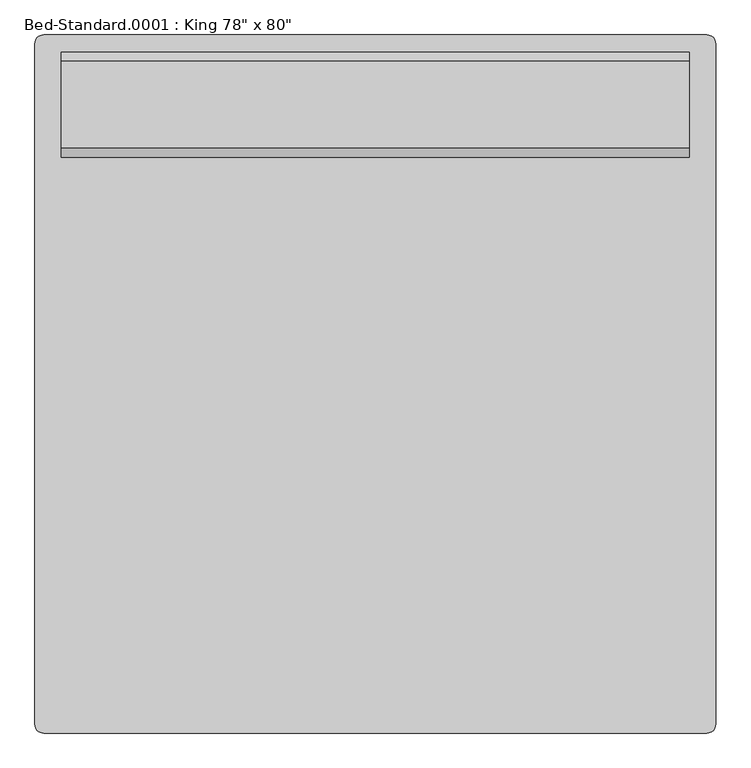
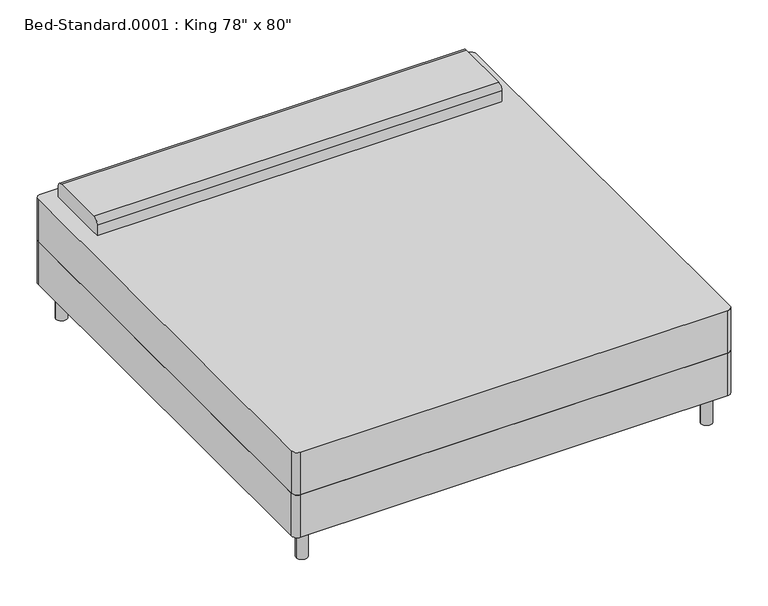
"""IFC4 building model written with IfcOpenShell, lengths in millimetres: furniture geometry."""

from ifc_helpers import new_model, si_unit, point, frame, frame_2d, origin, origin_with_axes, place, context, project, spatial, polyline, circle_curve, trimmed, segment, composite_curve, outline, extrude, source, transform, mapped, element, save


def furniture_1fc5af50(model_context):
    return source(origin(), model_context, "Body", "SweptSolid", [
        extrude(outline(composite_curve([segment(polyline([(-719.1114754, -1036.195082), (-719.1114754, 945.004918)]), True, "CONTINUOUS"), segment(trimmed(circle_curve(frame_2d((-693.7114754, 945.004918)), 25.4), [point((-719.1114754, 945.004918))], [point((-693.7114754, 970.404918))], False, "CARTESIAN"), True, "CONTINUOUS"), segment(polyline([(-693.7114754, 970.404918), (1236.6885246, 970.404918)]), True, "CONTINUOUS"), segment(trimmed(circle_curve(frame_2d((1236.6885246, 945.004918)), 25.4), [point((1236.6885246, 970.404918))], [point((1262.0885246, 945.004918))], False, "CARTESIAN"), True, "CONTINUOUS"), segment(polyline([(1262.0885246, 945.004918), (1262.0885246, -1036.195082)]), True, "CONTINUOUS"), segment(trimmed(circle_curve(frame_2d((1236.6885246, -1036.195082)), 25.4), [point((1262.0885246, -1036.195082))], [point((1236.6885246, -1061.595082))], False, "CARTESIAN"), True, "CONTINUOUS"), segment(polyline([(1236.6885246, -1061.595082), (-693.7114754, -1061.595082)]), True, "CONTINUOUS"), segment(trimmed(circle_curve(frame_2d((-693.7114754, -1036.195082)), 25.4), [point((-693.7114754, -1061.595082))], [point((-719.1114754, -1036.195082))], False, "CARTESIAN"), True, "CONTINUOUS")], self_intersect=False)), frame((0.0, 0.0, 152.4), z_axis=(0.0, 0.0, 1.0), x_axis=(1.0, 0.0, 0.0)), (0.0, 0.0, 1.0), 203.2),
        extrude(outline(composite_curve([segment(polyline([(614.804918, 558.8), (614.804918, 609.6)]), True, "CONTINUOUS"), segment(trimmed(circle_curve(frame_2d((640.204918, 609.6)), 25.4), [point((614.804918, 609.6))], [point((640.204918, 635.0))], False, "CARTESIAN"), True, "CONTINUOUS"), segment(polyline([(640.204918, 635.0), (894.204918, 635.0)]), True, "CONTINUOUS"), segment(trimmed(circle_curve(frame_2d((894.204918, 609.6)), 25.4), [point((894.204918, 635.0))], [point((919.604918, 609.6))], False, "CARTESIAN"), True, "CONTINUOUS"), segment(polyline([(919.604918, 609.6), (919.604918, 558.8), (614.804918, 558.8)]), True, "CONTINUOUS")], self_intersect=False)), frame((-642.9114754, 0.0, 0.0), z_axis=(1.0, 0.0, 0.0), x_axis=(0.0, 1.0, 0.0)), (0.0, 0.0, 1.0), 1828.8),
        extrude(outline(composite_curve([segment(trimmed(circle_curve(frame_2d((-642.9114754, 894.204918)), 25.4), [point((-668.3114754, 894.204918))], [point((-617.5114754, 894.204918))], False, "CARTESIAN"), True, "CONTINUOUS"), segment(trimmed(circle_curve(frame_2d((-642.9114754, 894.204918)), 25.4), [point((-617.5114754, 894.204918))], [point((-668.3114754, 894.204918))], False, "CARTESIAN"), True, "CONTINUOUS")], self_intersect=False)), origin_with_axes(), (0.0, 0.0, 1.0), 152.4),
        extrude(outline(composite_curve([segment(trimmed(circle_curve(frame_2d((1185.8885246, 894.204918)), 25.4), [point((1160.4885246, 894.204918))], [point((1211.2885246, 894.204918))], False, "CARTESIAN"), True, "CONTINUOUS"), segment(trimmed(circle_curve(frame_2d((1185.8885246, 894.204918)), 25.4), [point((1211.2885246, 894.204918))], [point((1160.4885246, 894.204918))], False, "CARTESIAN"), True, "CONTINUOUS")], self_intersect=False)), origin_with_axes(), (0.0, 0.0, 1.0), 152.4),
        extrude(outline(composite_curve([segment(trimmed(circle_curve(frame_2d((1185.8885246, -985.395082)), 25.4), [point((1160.4885246, -985.395082))], [point((1211.2885246, -985.395082))], False, "CARTESIAN"), True, "CONTINUOUS"), segment(trimmed(circle_curve(frame_2d((1185.8885246, -985.395082)), 25.4), [point((1211.2885246, -985.395082))], [point((1160.4885246, -985.395082))], False, "CARTESIAN"), True, "CONTINUOUS")], self_intersect=False)), origin_with_axes(), (0.0, 0.0, 1.0), 152.4),
        extrude(outline(composite_curve([segment(trimmed(circle_curve(frame_2d((-642.9114754, -985.395082)), 25.4), [point((-668.3114754, -985.395082))], [point((-617.5114754, -985.395082))], False, "CARTESIAN"), True, "CONTINUOUS"), segment(trimmed(circle_curve(frame_2d((-642.9114754, -985.395082)), 25.4), [point((-617.5114754, -985.395082))], [point((-668.3114754, -985.395082))], False, "CARTESIAN"), True, "CONTINUOUS")], self_intersect=False)), origin_with_axes(), (0.0, 0.0, 1.0), 152.4),
        extrude(outline(composite_curve([segment(polyline([(-693.7114754, 970.404918), (1236.6885246, 970.404918)]), True, "CONTINUOUS"), segment(trimmed(circle_curve(frame_2d((1236.6885246, 945.004918)), 25.4), [point((1236.6885246, 970.404918))], [point((1262.0885246, 945.004918))], False, "CARTESIAN"), True, "CONTINUOUS"), segment(polyline([(1262.0885246, 945.004918), (1262.0885246, -1036.195082)]), True, "CONTINUOUS"), segment(trimmed(circle_curve(frame_2d((1236.6885246, -1036.195082)), 25.4), [point((1262.0885246, -1036.195082))], [point((1236.6885246, -1061.595082))], False, "CARTESIAN"), True, "CONTINUOUS"), segment(polyline([(1236.6885246, -1061.595082), (-693.7114754, -1061.595082)]), True, "CONTINUOUS"), segment(trimmed(circle_curve(frame_2d((-693.7114754, -1036.195082)), 25.4), [point((-693.7114754, -1061.595082))], [point((-719.1114754, -1036.195082))], False, "CARTESIAN"), True, "CONTINUOUS"), segment(polyline([(-719.1114754, -1036.195082), (-719.1114754, 945.004918)]), True, "CONTINUOUS"), segment(trimmed(circle_curve(frame_2d((-693.7114754, 945.004918)), 25.4), [point((-719.1114754, 945.004918))], [point((-693.7114754, 970.404918))], False, "CARTESIAN"), True, "CONTINUOUS")], self_intersect=False)), frame((0.0, 0.0, 355.6), z_axis=(0.0, 0.0, 1.0), x_axis=(1.0, 0.0, 0.0)), (0.0, 0.0, 1.0), 203.2),
    ])


if __name__ == "__main__":
    model = new_model("IFC4")
    model_context = context("Model", 3, world=origin())
    ifc_project = project(units=[si_unit("LENGTHUNIT", "METRE", prefix="MILLI")], contexts=[model_context])
    site = spatial("IfcSite", under=ifc_project)
    building = spatial("IfcBuilding", under=site)
    placement = place(None, origin())
    furniture_shape = furniture_1fc5af50(model_context)
    element("IfcFurniture", 1, ObjectType="Bed-Standard.0001 : King 78\" x 80\"", at=placement, inside=building, context=model_context, shape_type="MappedRepresentation", body=[
        mapped(furniture_shape, transform((0.0, 0.0, 0.0), x_axis=(1.0, 0.0, 0.0), y_axis=(0.0, 1.0, 0.0), z_axis=(0.0, 0.0, 1.0))),
    ])
    save(model, "model.ifc")

# Revit data of these elements
# Type "Bed-Standard.0001 : King 78\" x 80\""
#   Assembly Code = "E2020200"
#   Length = 6' - 8"
#   Width = 6' - 6"
#   Leg Material = Steel, Chrome Plated
#   Mattress Material = Cherry
#   Default Elevation = 0
# Element 1 (IfcFurniture, "Bed-Standard.0001 : King 78\" x 80\"")
#   Materials on its faces: "Linen, White", "Steel, Chrome Plated"
# Materials
#   "Steel, Chrome Plated": class "Metal", colour RGB 17 17 17, transparency 0, Description = "Chromiuim plated steel", Cost = 0
#   "Cherry": class "Wood", colour RGB 226 177 128, transparency 0, Description = "Prunus Serotina", Cost = 0
#   "Linen, White": class "Textile", colour RGB 247 247 239, transparency 0, Description = "Linen, white", Cost = 0
